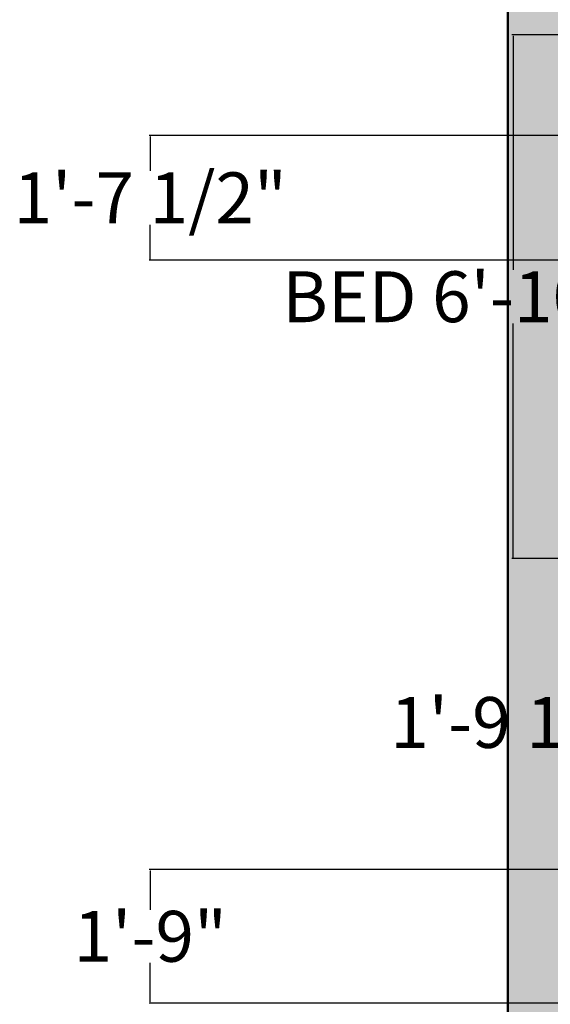
# Model space of a CAD drawing. Units: inches. Extents: x 22042254 to 25404563, y 17568978 to 17626777.
# Tile 38 of 45: x 22179707 to 22179790, y 17626539 to 17626694. Entities that reach past the tile are written whole.
import ezdxf

# ---------------------------------------------------------------- set-up
doc = ezdxf.new("R2010")
doc.units = ezdxf.units.IN
doc.header["$MEASUREMENT"] = 0
for name, color, linetype, lineweight in [('A-ANNO-DIMS', 2, 'Continuous', 18), ('A-WALL-PATT', 244, 'Continuous', 13), ('walls', 252, 'Continuous', 50)]:
    doc.layers.add(name, color=color, linetype=linetype, lineweight=lineweight)
doc.styles.get("Standard").update_dxf_attribs({"font": 'arial.ttf'})
doc.dimstyles.get("Standard").update_dxf_attribs({"dimtxt": 8, "dimasz": 0.18, "dimexe": 0.18, "dimexo": 0.0625, "dimgap": 0.09, "dimtad": 0, "dimtih": 1, "dimtoh": 1, "dimzin": 0, "dimdsep": 46, "dimlunit": 3, "dimtxsty": 'Standard', "dimcen": 0.09, "dimadec": 0, "dimazin": 0, "dimtfac": 1, "dimtofl": 0, "dimtmove": 0, "dimatfit": 3, "dimfxl": 1, "dimtolj": 1, "dimtzin": 0, "dimarcsym": 0})

# ---------------------------------------------------------------- blocks, each defined once
blk = doc.blocks.new('*D30')
at = {"layer": 'A-ANNO-DIMS', "color": 0, "lineweight": -2, "transparency": 16777216}
for p, q in [((22179796.84, 17626691.22), (22179784.37, 17626691.22)), ((22179784.55, 17626691.04), (22179784.55, 17626654.25)), ((22179784.55, 17626609.02), (22179784.55, 17626645.8)), ((22179796.84, 17626608.84), (22179784.37, 17626608.84))]:
    blk.add_line(p, q, dxfattribs=at)
at = {"layer": 'A-ANNO-DIMS', "color": 0, "transparency": 16777216}
for points in [[(22179784.52, 17626691.04), (22179784.58, 17626691.04), (22179784.55, 17626691.22)], [(22179784.52, 17626609.02), (22179784.58, 17626609.02), (22179784.55, 17626608.84)]]:
    blk.add_solid(points, dxfattribs=at)
at = {"layer": 'Defpoints', "color": 0, "transparency": 16777216}
for p in [(22179784.55, 17626691.22), (22179796.91, 17626691.22), (22179796.91, 17626608.84)]:
    blk.add_point(p, dxfattribs=at)
at = {"layer": 'A-ANNO-DIMS', "color": 0, "transparency": 16777216, "insert": (22179784.55, 17626650.03), "char_height": 8, "attachment_point": 5}
blk.add_mtext('\\A1;BED 6\'-10 1/2"', dxfattribs=at)
blk = doc.blocks.new('*D45')
at = {"layer": 'A-ANNO-DIMS', "color": 0, "lineweight": -2, "transparency": 16777216}
for p, q in [((22179832.67, 17626578.74), (22179832.67, 17626583.25)), ((22179854.32, 17626578.74), (22179854.32, 17626583.25)), ((22179832.67, 17626583.07), (22179832.49, 17626583.07)), ((22179854.14, 17626583.07), (22179832.85, 17626583.07))]:
    blk.add_line(p, q, dxfattribs=at)
at = {"layer": 'A-ANNO-DIMS', "color": 0, "transparency": 16777216}
for points in [[(22179832.85, 17626583.1), (22179832.85, 17626583.04), (22179832.67, 17626583.07)], [(22179854.14, 17626583.1), (22179854.14, 17626583.04), (22179854.32, 17626583.07)]]:
    blk.add_solid(points, dxfattribs=at)
at = {"layer": 'Defpoints', "color": 0, "transparency": 16777216}
for p in [(22179832.67, 17626583.07), (22179832.67, 17626578.68), (22179854.32, 17626578.68)]:
    blk.add_point(p, dxfattribs=at)
at = {"layer": 'A-ANNO-DIMS', "color": 0, "transparency": 16777216, "insert": (22179799.07, 17626583.07), "char_height": 8, "attachment_point": 5}
blk.add_mtext('\\A1;1\'-9 1/2" TYP.', dxfattribs=at)
blk = doc.blocks.new('*D61')
at = {"layer": 'A-ANNO-DIMS', "color": 0, "lineweight": -2, "transparency": 16777216}
for p, q in [((22179818.67, 17626559.94), (22179727.35, 17626559.94)), ((22179727.53, 17626559.76), (22179727.53, 17626553.61)), ((22179727.53, 17626539.12), (22179727.53, 17626545.26)), ((22179818.67, 17626538.94), (22179727.35, 17626538.94))]:
    blk.add_line(p, q, dxfattribs=at)
at = {"layer": 'A-ANNO-DIMS', "color": 0, "transparency": 16777216}
for points in [[(22179727.5, 17626559.76), (22179727.56, 17626559.76), (22179727.53, 17626559.94)], [(22179727.5, 17626539.12), (22179727.56, 17626539.12), (22179727.53, 17626538.94)]]:
    blk.add_solid(points, dxfattribs=at)
at = {"layer": 'Defpoints', "color": 0, "transparency": 16777216}
for p in [(22179818.73, 17626559.94), (22179727.53, 17626538.94), (22179818.73, 17626538.94)]:
    blk.add_point(p, dxfattribs=at)
at = {"layer": 'A-ANNO-DIMS', "color": 0, "transparency": 16777216, "insert": (22179727.53, 17626549.44), "char_height": 8, "attachment_point": 5}
blk.add_mtext('\\A1;1\'-9"', dxfattribs=at)
blk = doc.blocks.new('*D62')
at = {"layer": 'A-ANNO-DIMS', "color": 0, "lineweight": -2, "transparency": 16777216}
for p, q in [((22179965.84, 17626675.39), (22179727.35, 17626675.39)), ((22179727.53, 17626675.21), (22179727.53, 17626669.81)), ((22179727.53, 17626655.96), (22179727.53, 17626661.36)), ((22179962.16, 17626655.78), (22179727.35, 17626655.78))]:
    blk.add_line(p, q, dxfattribs=at)
at = {"layer": 'A-ANNO-DIMS', "color": 0, "transparency": 16777216}
for points in [[(22179727.5, 17626675.21), (22179727.56, 17626675.21), (22179727.53, 17626675.39)], [(22179727.5, 17626655.96), (22179727.56, 17626655.96), (22179727.53, 17626655.78)]]:
    blk.add_solid(points, dxfattribs=at)
at = {"layer": 'Defpoints', "color": 0, "transparency": 16777216}
for p in [(22179965.9, 17626675.39), (22179727.53, 17626655.78), (22179962.22, 17626655.78)]:
    blk.add_point(p, dxfattribs=at)
at = {"layer": 'A-ANNO-DIMS', "color": 0, "transparency": 16777216, "insert": (22179727.53, 17626665.59), "char_height": 8, "attachment_point": 5}
blk.add_mtext('\\A1;1\'-7 1/2"', dxfattribs=at)

msp = doc.modelspace()

# ---------------------------------------------------------------- hatches: boundary and pattern name
at = {"layer": 'A-WALL-PATT'}
h = msp.add_hatch(color=256, dxfattribs=at)
h.dxf.hatch_style = 1
h.paths.add_polyline_path([(22179792.734, 17626580.28), (22179888.734, 17626580.28), (22179888.734, 17626559.623), (22179893.234, 17626559.623), (22179893.234, 17626580.28), (22179900.438, 17626580.28), (22179900.438, 17626584.78), (22179792.734, 17626584.78), (22179792.734, 17626728.78), (22180134.734, 17626728.78), (22180134.734, 17626584.78), (22180035.602, 17626584.78), (22180004.432, 17626584.78), (22180001.734, 17626584.78), (22180001.734, 17626580.28), (22180134.734, 17626580.28), (22180134.734, 17626404.28), (22180064.487, 17626404.28), (22180064.487, 17626399.78), (22180134.734, 17626399.78), (22180134.734, 17626197.78), (22180143.734, 17626197.78), (22180143.734, 17626737.78), (22179783.734, 17626737.78), (22179783.734, 17626197.78), (22179792.734, 17626197.78), (22179792.734, 17626394.78), (22179936.734, 17626394.78), (22179936.734, 17626383.208), (22179941.234, 17626383.208), (22179941.234, 17626532.28), (22179927.066, 17626532.28), (22179927.066, 17626527.78), (22179928.072, 17626527.78), (22179936.734, 17626527.78), (22179936.734, 17626403.78), (22179792.734, 17626403.78), (22179792.734, 17626527.78), (22179905.094, 17626527.78), (22179905.094, 17626532.28), (22179792.734, 17626532.28)])

# ---------------------------------------------------------------- linework, layer by layer
at = {"layer": 'walls'}
msp.add_line((22179783.734, 17626197.78), (22179783.734, 17626737.78), dxfattribs=at)

# ---------------------------------------------------------------- dimensions: what is measured, and where the dimension line sits
at = {"layer": 'A-ANNO-DIMS'}
for base, p1, p2, angle, text, picture, middle in [((22179784.549, 17626691.22), (22179796.907, 17626608.836), (22179796.907, 17626691.22), 90, 'BED <>', '*D30', (22179784.549, 17626650.028)), ((22179832.666, 17626583.067), (22179854.322, 17626578.675), (22179832.666, 17626578.675), 180, '<> TYP.', '*D45', (22179799.07, 17626583.067))]:
    dim = msp.add_linear_dim(base=base, p1=p1, p2=p2, angle=angle, text=text, dimstyle='Standard', override={"dimdec": 1, "dimlfac": 1, "dimrnd": 0, "dimzin": 1, "dimdsep": 46, "dimlunit": 4, "dimfrac": 2}, dxfattribs=at)
    dim.commit()
    dim.dimension.update_dxf_attribs({"geometry": picture, "text_midpoint": middle})
for base, p1, p2, picture, middle in [((22179727.534, 17626655.782), (22179965.901, 17626675.394), (22179962.224, 17626655.782), '*D62', (22179727.534, 17626665.588)), ((22179727.534, 17626538.936), (22179818.734, 17626559.936), (22179818.734, 17626538.936), '*D61', (22179727.534, 17626549.436))]:
    dim = msp.add_linear_dim(base=base, p1=p1, p2=p2, angle=90, dimstyle='Standard', override={"dimdec": 1, "dimlfac": 1, "dimrnd": 0, "dimzin": 1, "dimdsep": 46, "dimlunit": 4, "dimfrac": 2}, dxfattribs=at)
    dim.commit()
    dim.dimension.update_dxf_attribs({"geometry": picture, "text_midpoint": middle})

doc.saveas('drawing.dxf')
